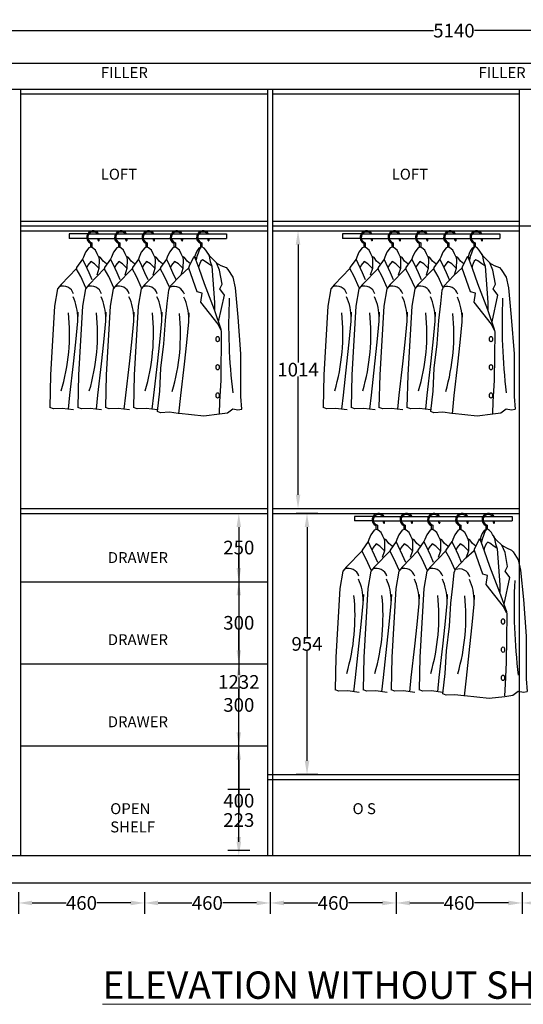
# Model space of a CAD drawing. Units: millimetres. Extents: x -472 to 16192, y -4730 to 4331.
# Tile 5 of 8: x 10934 to 12774, y -4730 to -1132. Entities that reach past the tile are written whole.
import ezdxf

# ---------------------------------------------------------------- set-up
doc = ezdxf.new("R2010")
doc.units = ezdxf.units.MM
doc.header["$MEASUREMENT"] = 0
for name, color, linetype, lineweight in [('A-ANNO-DIMS', 2, 'Continuous', 18), ('A-ANNO-TEXT', 6, 'Continuous', 18), ('A-ELEV', 7, 'Continuous', 25), ('A-FURN', 8, 'Continuous', 25)]:
    doc.layers.add(name, color=color, linetype=linetype, lineweight=lineweight)
doc.styles.get("Standard").update_dxf_attribs({"font": 'arial.ttf'})
doc.dimstyles.get("Standard").update_dxf_attribs({"dimtxt": 50, "dimasz": 50, "dimexe": 40, "dimexo": 40, "dimgap": 0.09, "dimtad": 0, "dimtih": 1, "dimtoh": 1, "dimdec": 0, "dimzin": 0, "dimdsep": 46, "dimtxsty": 'Standard', "dimcen": 0.09, "dimclrd": 1, "dimclre": 3, "dimclrt": 6, "dimadec": 0, "dimazin": 0, "dimtfac": 1, "dimtdec": 0, "dimtofl": 0, "dimtmove": 0, "dimatfit": 3, "dimfxl": 40, "dimfxlon": 1, "dimtolj": 1, "dimtzin": 0, "dimarcsym": 0})

# ---------------------------------------------------------------- blocks, each defined once
blk = doc.blocks.new('*D44')
at = {"layer": 'A-ANNO-DIMS', "color": 0, "lineweight": -2, "transparency": 16777216}
for p, q in [((9950.7, -1212.4), (9950.7, -1132.4)), ((15090.7, -1212.4), (15090.7, -1132.4)), ((10000.7, -1172.4), (12446, -1172.4)), ((15040.7, -1172.4), (12595.3, -1172.4))]:
    blk.add_line(p, q, dxfattribs=at)
at = {"layer": 'A-ANNO-DIMS', "color": 0, "transparency": 16777216}
for points in [[(10000.7, -1164.1), (10000.7, -1180.8), (9950.7, -1172.4)], [(15040.7, -1164.1), (15040.7, -1180.8), (15090.7, -1172.4)]]:
    blk.add_solid(points, dxfattribs=at)
at = {"layer": 'Defpoints', "color": 0, "transparency": 16777216}
for p in [(15090.7, -1172.4), (9950.7, -1290.9), (15090.7, -1290.9)]:
    blk.add_point(p, dxfattribs=at)
at = {"layer": 'A-ANNO-DIMS', "color": 0, "transparency": 16777216, "insert": (12520.7, -1172.4), "char_height": 50, "attachment_point": 5}
blk.add_mtext('\\A1;5140', dxfattribs=at)
blk = doc.blocks.new('*D54')
at = {"layer": 'A-ANNO-DIMS', "color": 0, "lineweight": -2, "transparency": 16777216}
for p, q in [((10929.7, -4319.4), (10929.7, -4399.4)), ((11389.7, -4319.4), (11389.7, -4399.4)), ((10979.7, -4359.4), (11103.4, -4359.4)), ((11339.7, -4359.4), (11215.9, -4359.4))]:
    blk.add_line(p, q, dxfattribs=at)
at = {"layer": 'A-ANNO-DIMS', "color": 0, "transparency": 16777216}
for points in [[(10979.7, -4351), (10979.7, -4367.7), (10929.7, -4359.4)], [(11339.7, -4351), (11339.7, -4367.7), (11389.7, -4359.4)]]:
    blk.add_solid(points, dxfattribs=at)
at = {"layer": 'Defpoints', "color": 0, "transparency": 16777216}
for p in [(10929.7, -4185.9), (11389.7, -4185.9), (11389.7, -4359.4)]:
    blk.add_point(p, dxfattribs=at)
at = {"layer": 'A-ANNO-DIMS', "color": 0, "transparency": 16777216, "insert": (11159.7, -4359.4), "char_height": 50, "attachment_point": 5}
blk.add_mtext('\\A1;460', dxfattribs=at)
blk = doc.blocks.new('*D55')
at = {"layer": 'A-ANNO-DIMS', "color": 0, "lineweight": -2, "transparency": 16777216}
for p, q in [((11389.7, -4319.4), (11389.7, -4399.4)), ((11849.7, -4319.4), (11849.7, -4399.4)), ((11439.7, -4359.4), (11563.4, -4359.4)), ((11799.7, -4359.4), (11675.9, -4359.4))]:
    blk.add_line(p, q, dxfattribs=at)
at = {"layer": 'A-ANNO-DIMS', "color": 0, "transparency": 16777216}
for points in [[(11439.7, -4351), (11439.7, -4367.7), (11389.7, -4359.4)], [(11799.7, -4351), (11799.7, -4367.7), (11849.7, -4359.4)]]:
    blk.add_solid(points, dxfattribs=at)
at = {"layer": 'Defpoints', "color": 0, "transparency": 16777216}
for p in [(11389.7, -4185.9), (11849.7, -4185.9), (11849.7, -4359.4)]:
    blk.add_point(p, dxfattribs=at)
at = {"layer": 'A-ANNO-DIMS', "color": 0, "transparency": 16777216, "insert": (11619.7, -4359.4), "char_height": 50, "attachment_point": 5}
blk.add_mtext('\\A1;460', dxfattribs=at)
blk = doc.blocks.new('*D56')
at = {"layer": 'A-ANNO-DIMS', "color": 0, "lineweight": -2, "transparency": 16777216}
for p, q in [((11849.7, -4319.4), (11849.7, -4399.4)), ((12309.7, -4319.4), (12309.7, -4399.4)), ((11899.7, -4359.4), (12023.4, -4359.4)), ((12259.7, -4359.4), (12135.9, -4359.4))]:
    blk.add_line(p, q, dxfattribs=at)
at = {"layer": 'A-ANNO-DIMS', "color": 0, "transparency": 16777216}
for points in [[(11899.7, -4351), (11899.7, -4367.7), (11849.7, -4359.4)], [(12259.7, -4351), (12259.7, -4367.7), (12309.7, -4359.4)]]:
    blk.add_solid(points, dxfattribs=at)
at = {"layer": 'Defpoints', "color": 0, "transparency": 16777216}
for p in [(11849.7, -4185.9), (12309.7, -4185.9), (12309.7, -4359.4)]:
    blk.add_point(p, dxfattribs=at)
at = {"layer": 'A-ANNO-DIMS', "color": 0, "transparency": 16777216, "insert": (12079.7, -4359.4), "char_height": 50, "attachment_point": 5}
blk.add_mtext('\\A1;460', dxfattribs=at)
blk = doc.blocks.new('*D57')
at = {"layer": 'A-ANNO-DIMS', "color": 0, "lineweight": -2, "transparency": 16777216}
for p, q in [((12309.7, -4319.4), (12309.7, -4399.4)), ((12769.7, -4319.4), (12769.7, -4399.4)), ((12359.7, -4359.4), (12483.4, -4359.4)), ((12719.7, -4359.4), (12595.9, -4359.4))]:
    blk.add_line(p, q, dxfattribs=at)
at = {"layer": 'A-ANNO-DIMS', "color": 0, "transparency": 16777216}
for points in [[(12359.7, -4351), (12359.7, -4367.7), (12309.7, -4359.4)], [(12719.7, -4351), (12719.7, -4367.7), (12769.7, -4359.4)]]:
    blk.add_solid(points, dxfattribs=at)
at = {"layer": 'Defpoints', "color": 0, "transparency": 16777216}
for p in [(12309.7, -4185.9), (12769.7, -4185.9), (12769.7, -4359.4)]:
    blk.add_point(p, dxfattribs=at)
at = {"layer": 'A-ANNO-DIMS', "color": 0, "transparency": 16777216, "insert": (12539.7, -4359.4), "char_height": 50, "attachment_point": 5}
blk.add_mtext('\\A1;460', dxfattribs=at)
blk = doc.blocks.new('*D58')
at = {"layer": 'A-ANNO-DIMS', "color": 0, "lineweight": -2, "transparency": 16777216}
for p, q in [((12769.7, -4319.4), (12769.7, -4399.4)), ((13229.7, -4319.4), (13229.7, -4399.4)), ((12819.7, -4359.4), (12943.4, -4359.4)), ((13179.7, -4359.4), (13055.9, -4359.4))]:
    blk.add_line(p, q, dxfattribs=at)
at = {"layer": 'A-ANNO-DIMS', "color": 0, "transparency": 16777216}
for points in [[(12819.7, -4351), (12819.7, -4367.7), (12769.7, -4359.4)], [(13179.7, -4351), (13179.7, -4367.7), (13229.7, -4359.4)]]:
    blk.add_solid(points, dxfattribs=at)
at = {"layer": 'Defpoints', "color": 0, "transparency": 16777216}
for p in [(12769.7, -4185.9), (13229.7, -4185.9), (13229.7, -4359.4)]:
    blk.add_point(p, dxfattribs=at)
at = {"layer": 'A-ANNO-DIMS', "color": 0, "transparency": 16777216, "insert": (12999.7, -4359.4), "char_height": 50, "attachment_point": 5}
blk.add_mtext('\\A1;460', dxfattribs=at)
blk = doc.blocks.new('*D73')
at = {"layer": 'A-ANNO-DIMS', "color": 0, "lineweight": -2, "transparency": 16777216}
for p, q in [((11911.1, -1903.9), (11991.1, -1903.9)), ((11951.1, -1953.9), (11951.1, -2385.3)), ((11951.1, -2867.9), (11951.1, -2436.5)), ((11911.1, -2917.9), (11991.1, -2917.9))]:
    blk.add_line(p, q, dxfattribs=at)
at = {"layer": 'A-ANNO-DIMS', "color": 0, "transparency": 16777216}
for points in [[(11942.8, -1953.9), (11959.5, -1953.9), (11951.1, -1903.9)], [(11942.8, -2867.9), (11959.5, -2867.9), (11951.1, -2917.9)]]:
    blk.add_solid(points, dxfattribs=at)
at = {"layer": 'Defpoints', "color": 0, "transparency": 16777216}
for p in [(11851.5, -1903.9), (11851.5, -2917.9), (11951.1, -2917.9)]:
    blk.add_point(p, dxfattribs=at)
at = {"layer": 'A-ANNO-DIMS', "color": 0, "transparency": 16777216, "insert": (11951.1, -2410.9), "char_height": 50, "attachment_point": 5}
blk.add_mtext('\\A1;1014', dxfattribs=at)
blk = doc.blocks.new('*D74')
at = {"layer": 'A-ANNO-DIMS', "color": 0, "lineweight": -2, "transparency": 16777216}
for p, q in [((12023.9, -2935.9), (11943.9, -2935.9)), ((11983.9, -2985.9), (11983.9, -3387.3)), ((11983.9, -3839.9), (11983.9, -3438.5)), ((12023.9, -3889.9), (11943.9, -3889.9))]:
    blk.add_line(p, q, dxfattribs=at)
at = {"layer": 'A-ANNO-DIMS', "color": 0, "transparency": 16777216}
for points in [[(11975.6, -2985.9), (11992.3, -2985.9), (11983.9, -2935.9)], [(11975.6, -3839.9), (11992.3, -3839.9), (11983.9, -3889.9)]]:
    blk.add_solid(points, dxfattribs=at)
at = {"layer": 'Defpoints', "color": 0, "transparency": 16777216}
for p in [(12121.2, -2935.9), (11983.9, -3889.9), (12103.5, -3889.9)]:
    blk.add_point(p, dxfattribs=at)
at = {"layer": 'A-ANNO-DIMS', "color": 0, "transparency": 16777216, "insert": (11983.9, -3412.9), "char_height": 50, "attachment_point": 5}
blk.add_mtext('\\A1;954', dxfattribs=at)
blk = doc.blocks.new('*D82')
at = {"layer": 'A-ANNO-DIMS', "color": 0, "lineweight": -2, "transparency": 16777216}
for p, q in [((11733.2, -3785.9), (11774.7, -3785.9)), ((11734.7, -3835.9), (11734.7, -3960.3)), ((11734.7, -4135.9), (11734.7, -4011.5)), ((11733.2, -4185.9), (11774.7, -4185.9))]:
    blk.add_line(p, q, dxfattribs=at)
at = {"layer": 'A-ANNO-DIMS', "color": 0, "transparency": 16777216}
for points in [[(11726.4, -3835.9), (11743, -3835.9), (11734.7, -3785.9)], [(11726.4, -4135.9), (11743, -4135.9), (11734.7, -4185.9)]]:
    blk.add_solid(points, dxfattribs=at)
at = {"layer": 'Defpoints', "color": 0, "transparency": 16777216}
for p in [(11693.2, -3785.9), (11734.7, -3785.9), (11693.2, -4185.9)]:
    blk.add_point(p, dxfattribs=at)
at = {"layer": 'A-ANNO-DIMS', "color": 0, "transparency": 16777216, "insert": (11734.7, -3985.9), "char_height": 50, "attachment_point": 5}
blk.add_mtext('\\A1;400', dxfattribs=at)
blk = doc.blocks.new('*D83')
at = {"layer": 'A-ANNO-DIMS', "color": 0, "lineweight": -2, "transparency": 16777216}
for p, q in [((11734.7, -3485.9), (11774.7, -3485.9)), ((11734.7, -3535.9), (11734.7, -3610.3)), ((11734.7, -3735.9), (11734.7, -3661.5)), ((11733.2, -3785.9), (11774.7, -3785.9))]:
    blk.add_line(p, q, dxfattribs=at)
at = {"layer": 'A-ANNO-DIMS', "color": 0, "transparency": 16777216}
for points in [[(11726.4, -3535.9), (11743, -3535.9), (11734.7, -3485.9)], [(11726.4, -3735.9), (11743, -3735.9), (11734.7, -3785.9)]]:
    blk.add_solid(points, dxfattribs=at)
at = {"layer": 'Defpoints', "color": 0, "transparency": 16777216}
for p in [(11734.7, -3485.9), (11734.7, -3485.9), (11693.2, -3785.9)]:
    blk.add_point(p, dxfattribs=at)
at = {"layer": 'A-ANNO-DIMS', "color": 0, "transparency": 16777216, "insert": (11734.7, -3635.9), "char_height": 50, "attachment_point": 5}
blk.add_mtext('\\A1;300', dxfattribs=at)
blk = doc.blocks.new('*D84')
at = {"layer": 'A-ANNO-DIMS', "color": 0, "lineweight": -2, "transparency": 16777216}
for p, q in [((11734.7, -3185.9), (11774.7, -3185.9)), ((11734.7, -3235.9), (11734.7, -3310.3)), ((11734.7, -3435.9), (11734.7, -3361.5)), ((11734.7, -3485.9), (11774.7, -3485.9))]:
    blk.add_line(p, q, dxfattribs=at)
at = {"layer": 'A-ANNO-DIMS', "color": 0, "transparency": 16777216}
for points in [[(11726.4, -3235.9), (11743, -3235.9), (11734.7, -3185.9)], [(11726.4, -3435.9), (11743, -3435.9), (11734.7, -3485.9)]]:
    blk.add_solid(points, dxfattribs=at)
at = {"layer": 'Defpoints', "color": 0, "transparency": 16777216}
for p in [(11734.7, -3185.9), (11734.7, -3185.9), (11734.7, -3485.9)]:
    blk.add_point(p, dxfattribs=at)
at = {"layer": 'A-ANNO-DIMS', "color": 0, "transparency": 16777216, "insert": (11734.7, -3335.9), "char_height": 50, "attachment_point": 5}
blk.add_mtext('\\A1;300', dxfattribs=at)
blk = doc.blocks.new('*D85')
at = {"layer": 'A-ANNO-DIMS', "color": 0, "lineweight": -2, "transparency": 16777216}
for p, q in [((11734.7, -2935.9), (11774.7, -2935.9)), ((11734.7, -2985.9), (11734.7, -3035.3)), ((11734.7, -3135.9), (11734.7, -3086.5)), ((11734.7, -3185.9), (11774.7, -3185.9))]:
    blk.add_line(p, q, dxfattribs=at)
at = {"layer": 'A-ANNO-DIMS', "color": 0, "transparency": 16777216}
for points in [[(11726.4, -2985.9), (11743, -2985.9), (11734.7, -2935.9)], [(11726.4, -3135.9), (11743, -3135.9), (11734.7, -3185.9)]]:
    blk.add_solid(points, dxfattribs=at)
at = {"layer": 'Defpoints', "color": 0, "transparency": 16777216}
for p in [(11734.7, -2935.9), (11734.7, -2935.9), (11734.7, -3185.9)]:
    blk.add_point(p, dxfattribs=at)
at = {"layer": 'A-ANNO-DIMS', "color": 0, "transparency": 16777216, "insert": (11734.7, -3060.9), "char_height": 50, "attachment_point": 5}
blk.add_mtext('\\A1;250', dxfattribs=at)
blk = doc.blocks.new('*D86')
at = {"layer": 'A-ANNO-DIMS', "color": 0, "lineweight": -2, "transparency": 16777216}
for p, q in [((11734.7, -2935.9), (11774.7, -2935.9)), ((11734.7, -2985.9), (11734.7, -3526.3)), ((11734.7, -4117.9), (11734.7, -3577.5)), ((11774.7, -4167.9), (11694.7, -4167.9))]:
    blk.add_line(p, q, dxfattribs=at)
at = {"layer": 'A-ANNO-DIMS', "color": 0, "transparency": 16777216}
for points in [[(11726.4, -2985.9), (11743, -2985.9), (11734.7, -2935.9)], [(11726.4, -4117.9), (11743, -4117.9), (11734.7, -4167.9)]]:
    blk.add_solid(points, dxfattribs=at)
at = {"layer": 'Defpoints', "color": 0, "transparency": 16777216}
for p in [(11734.7, -2935.9), (11734.7, -4167.9), (14004.4, -4167.9)]:
    blk.add_point(p, dxfattribs=at)
at = {"layer": 'A-ANNO-DIMS', "color": 0, "transparency": 16777216, "insert": (11734.7, -3551.9), "char_height": 50, "attachment_point": 5}
blk.add_mtext('\\A1;1232', dxfattribs=at)
blk = doc.blocks.new('*D87')
at = {"layer": 'A-ANNO-DIMS', "color": 0, "lineweight": -2, "transparency": 16777216}
for p, q in [((11774.7, -3944.9), (11694.7, -3944.9)), ((11734.7, -3994.9), (11734.7, -4030.8)), ((11734.7, -4117.9), (11734.7, -4082)), ((11774.7, -4167.9), (11694.7, -4167.9))]:
    blk.add_line(p, q, dxfattribs=at)
at = {"layer": 'A-ANNO-DIMS', "color": 0, "transparency": 16777216}
for points in [[(11726.4, -3994.9), (11743, -3994.9), (11734.7, -3944.9)], [(11726.4, -4117.9), (11743, -4117.9), (11734.7, -4167.9)]]:
    blk.add_solid(points, dxfattribs=at)
at = {"layer": 'Defpoints', "color": 0, "transparency": 16777216}
for p in [(11734.7, -3944.9), (13999.1, -3944.9), (14004.4, -4167.9)]:
    blk.add_point(p, dxfattribs=at)
at = {"layer": 'A-ANNO-DIMS', "color": 0, "transparency": 16777216, "insert": (11734.7, -4056.4), "char_height": 50, "attachment_point": 5}
blk.add_mtext('\\A1;223', dxfattribs=at)
blk = doc.blocks.new('7')
for p, q in [((3901.77, 12903.37), (3898.37, 12903.37)), ((3898.37, 12903.37), (3898.37, 12902.56)), ((3901.6, 12902.56), (3898.37, 12902.56)), ((3901.81, 12902.56), (3906.72, 12902.56)), ((3902.01, 12903.37), (3906.88, 12903.37)), ((3902.55, 12901.75), (3902.55, 12900.89)), ((3903.8, 12903.37), (3905.4, 12903.37)), ((3906.93, 12902.56), (3911.77, 12902.56)), ((3907.13, 12903.37), (3911.93, 12903.37)), ((3907.67, 12901.75), (3907.67, 12900.89)), ((3911.97, 12902.56), (3916.93, 12902.56)), ((3912.18, 12903.37), (3917.09, 12903.37)), ((3912.72, 12901.75), (3912.72, 12900.89)), ((3917.13, 12902.56), (3921.77, 12902.56)), ((3917.33, 12903.37), (3921.94, 12903.37)), ((3917.87, 12901.75), (3917.87, 12900.92)), ((3921.98, 12902.56), (3927.26, 12902.56)), ((3922.18, 12903.37), (3927.26, 12903.37)), ((3922.72, 12901.75), (3922.72, 12901.02)), ((3927.26, 12903.37), (3927.26, 12902.56)), ((3901.37, 12900), (3900.98, 12899.12)), ((3901.99, 12900.85), (3901.37, 12900)), ((3902.38, 12900.93), (3901.99, 12900.85)), ((3902.35, 12900.89), (3902.35, 12901.61)), ((3902.69, 12900.85), (3902.38, 12900.93)), ((3903.23, 12900.39), (3902.69, 12900.85)), ((3903.54, 12899.74), (3903.23, 12900.39)), ((3906.51, 12900), (3906.12, 12899.12)), ((3907.13, 12900.85), (3906.51, 12900)), ((3907.52, 12900.93), (3907.13, 12900.85)), ((3907.47, 12900.89), (3907.47, 12901.61)), ((3907.83, 12900.85), (3907.52, 12900.93)), ((3908.37, 12900.39), (3907.83, 12900.85)), ((3908.68, 12899.74), (3908.37, 12900.39)), ((3911.62, 12900), (3911.24, 12899.12)), ((3912.25, 12900.85), (3911.62, 12900)), ((3912.63, 12900.93), (3912.25, 12900.85)), ((3912.51, 12900.89), (3912.51, 12901.61)), ((3912.94, 12900.85), (3912.63, 12900.93)), ((3913.49, 12900.39), (3912.94, 12900.85)), ((3913.8, 12899.74), (3913.49, 12900.39)), ((3916.76, 12900), (3916.38, 12899.12)), ((3917.39, 12900.85), (3916.76, 12900)), ((3917.77, 12900.93), (3917.39, 12900.85)), ((3917.67, 12900.91), (3917.67, 12901.61)), ((3918.08, 12900.85), (3917.77, 12900.93)), ((3918.63, 12900.39), (3918.08, 12900.85)), ((3918.94, 12899.74), (3918.63, 12900.39)), ((3921.8, 12900.21), (3921.6, 12899.78)), ((3922.16, 12900.76), (3921.8, 12900.21)), ((3922.35, 12900.7), (3922.02, 12899.87)), ((3922.57, 12901.03), (3922.16, 12900.76)), ((3922.57, 12901.03), (3922.35, 12900.7)), ((3922.52, 12901), (3922.52, 12901.61)), ((3922.75, 12901), (3922.57, 12901.03)), ((3923.13, 12900.79), (3922.75, 12901)), ((3923.47, 12900.38), (3923.13, 12900.79)), ((3923.71, 12900.01), (3923.47, 12900.38)), ((3924, 12899.6), (3923.71, 12900.01)), ((3900.85, 12898.74), (3899.74, 12897.19)), ((3900.98, 12899.12), (3900.85, 12898.73)), ((3901.25, 12897.93), (3900.85, 12898.74)), ((3902.33, 12898.32), (3901.78, 12897.67)), ((3903.03, 12897.88), (3902.33, 12898.32)), ((3903.78, 12899.26), (3903.54, 12899.74)), ((3904.15, 12899.04), (3903.78, 12899.26)), ((3903.78, 12899.26), (3903.89, 12898.71)), ((3903.89, 12898.71), (3903.85, 12897.04)), ((3904.63, 12898.37), (3904.15, 12899.04)), ((3905.24, 12897.91), (3904.63, 12898.37)), ((3905.99, 12898.74), (3904.88, 12897.19)), ((3906.12, 12899.12), (3905.99, 12898.73)), ((3906.39, 12897.93), (3905.99, 12898.74)), ((3907.47, 12898.32), (3906.92, 12897.67)), ((3908.17, 12897.88), (3907.47, 12898.32)), ((3908.92, 12899.26), (3908.68, 12899.74)), ((3909.29, 12899.04), (3908.92, 12899.26)), ((3908.92, 12899.26), (3909.03, 12898.71)), ((3909.03, 12898.71), (3908.99, 12897.04)), ((3909.77, 12898.37), (3909.29, 12899.04)), ((3910.38, 12897.91), (3909.77, 12898.37)), ((3911.1, 12898.74), (3909.99, 12897.19)), ((3911.51, 12897.93), (3911.1, 12898.74)), ((3911.24, 12899.12), (3911.11, 12898.73)), ((3912.58, 12898.32), (3912.04, 12897.67)), ((3913.28, 12897.88), (3912.58, 12898.32)), ((3914.03, 12899.26), (3913.8, 12899.74)), ((3914.4, 12899.04), (3914.03, 12899.26)), ((3914.03, 12899.26), (3914.14, 12898.71)), ((3914.14, 12898.71), (3914.11, 12897.04)), ((3914.88, 12898.37), (3914.4, 12899.04)), ((3915.5, 12897.91), (3914.88, 12898.37)), ((3916.24, 12898.74), (3915.13, 12897.19)), ((3916.65, 12897.93), (3916.24, 12898.74)), ((3916.38, 12899.12), (3916.25, 12898.73)), ((3917.72, 12898.32), (3917.18, 12897.67)), ((3918.42, 12897.88), (3917.72, 12898.32)), ((3919.17, 12899.26), (3918.94, 12899.74)), ((3919.54, 12899.04), (3919.17, 12899.26)), ((3919.17, 12899.26), (3919.28, 12898.71)), ((3919.28, 12898.71), (3919.25, 12897.04)), ((3920.02, 12898.37), (3919.54, 12899.04)), ((3920.64, 12897.91), (3920.02, 12898.37)), ((3920.43, 12897.51), (3920.79, 12898.19)), ((3920.79, 12898.19), (3921.19, 12898.97)), ((3921.19, 12898.97), (3921.35, 12899.23)), ((3921.3, 12899.16), (3921.61, 12898.57)), ((3921.35, 12899.23), (3921.7, 12898.97)), ((3921.6, 12899.78), (3921.4, 12899.16)), ((3921.61, 12898.57), (3922.15, 12897.07)), ((3921.66, 12898.64), (3921.65, 12898.56)), ((3921.8, 12899.21), (3921.66, 12898.64)), ((3921.7, 12898.97), (3921.75, 12898.95)), ((3922.02, 12899.87), (3921.8, 12899.21)), ((3922.55, 12898.4), (3922.33, 12897.95)), ((3922.82, 12898.65), (3922.55, 12898.4)), ((3923.17, 12898.44), (3922.82, 12898.65)), ((3923.96, 12897.86), (3923.17, 12898.44)), ((3924.38, 12899.09), (3923.92, 12899.61)), ((3924, 12899.6), (3924.26, 12898.31)), ((3924.26, 12898.31), (3924.56, 12897.43)), ((3925.4, 12898.1), (3924.38, 12899.09)), ((3899.74, 12897.04), (3896.88, 12894.08)), ((3900.49, 12895.54), (3899.68, 12897.02)), ((3899.74, 12897.19), (3899.74, 12897.04)), ((3902.03, 12896.26), (3901.25, 12897.93)), ((3901.78, 12897.67), (3901.59, 12897.2)), ((3904.88, 12897.04), (3902.02, 12894.08)), ((3903.88, 12897.03), (3903.03, 12897.88)), ((3903.85, 12897.04), (3903.46, 12895.81)), ((3905.63, 12895.54), (3904.82, 12897.02)), ((3904.88, 12897.19), (3904.88, 12897.04)), ((3907.17, 12896.26), (3906.39, 12897.93)), ((3906.92, 12897.67), (3906.73, 12897.2)), ((3909.99, 12897.04), (3907.14, 12894.08)), ((3909.02, 12897.03), (3908.17, 12897.88)), ((3908.99, 12897.04), (3908.6, 12895.81)), ((3910.75, 12895.54), (3909.93, 12897.02)), ((3909.99, 12897.19), (3909.99, 12897.04)), ((3912.29, 12896.26), (3911.51, 12897.93)), ((3912.04, 12897.67), (3911.85, 12897.2)), ((3915.13, 12897.04), (3912.28, 12894.08)), ((3914.13, 12897.03), (3913.28, 12897.88)), ((3914.11, 12897.04), (3913.72, 12895.81)), ((3915.89, 12895.54), (3915.07, 12897.02)), ((3915.13, 12897.19), (3915.13, 12897.04)), ((3917.43, 12896.26), (3916.65, 12897.93)), ((3917.18, 12897.67), (3916.99, 12897.2)), ((3919.27, 12897.03), (3918.42, 12897.88)), ((3918.8, 12895.75), (3920.32, 12897.13)), ((3919.25, 12897.04), (3918.86, 12895.81)), ((3920.32, 12897.13), (3920.43, 12897.51)), ((3921.88, 12892.78), (3920.35, 12897.12)), ((3922.18, 12897.46), (3922.13, 12897.29)), ((3922.15, 12897.07), (3923.16, 12894.25)), ((3922.33, 12897.95), (3922.18, 12897.46)), ((3924.48, 12897.51), (3923.96, 12897.86)), ((3924.56, 12897.43), (3925.04, 12890.79)), ((3925.37, 12898.1), (3926.22, 12897.58)), ((3925.98, 12896.74), (3925.4, 12898.1)), ((3926.43, 12894.14), (3925.98, 12896.74)), ((3926.22, 12897.58), (3927.16, 12897.19)), ((3927.16, 12897.19), (3927.49, 12896.83)), ((3927.49, 12896.83), (3928.42, 12895.42)), ((3901.42, 12893.5), (3900.49, 12895.54)), ((3902.61, 12894.93), (3902.03, 12896.26)), ((3906.56, 12893.5), (3905.63, 12895.54)), ((3907.75, 12894.93), (3907.17, 12896.26)), ((3911.68, 12893.5), (3910.75, 12895.54)), ((3912.86, 12894.93), (3912.29, 12896.26)), ((3916.82, 12893.5), (3915.89, 12895.54)), ((3916.93, 12893.82), (3918.8, 12895.75)), ((3918, 12894.93), (3917.43, 12896.26)), ((3928.42, 12895.42), (3928.82, 12893.49)), ((3896.21, 12893.3), (3895.68, 12890.13)), ((3896.88, 12894.08), (3896.21, 12893.3)), ((3901.35, 12893.3), (3900.82, 12890.13)), ((3902.02, 12894.08), (3901.35, 12893.3)), ((3906.47, 12893.3), (3905.93, 12890.13)), ((3907.14, 12894.08), (3906.47, 12893.3)), ((3911.61, 12893.3), (3911.07, 12890.13)), ((3912.28, 12894.08), (3911.61, 12893.3)), ((3916.38, 12890.58), (3916.66, 12893.06)), ((3916.66, 12893.06), (3916.93, 12893.82)), ((3922.78, 12892.51), (3921.88, 12892.78)), ((3923.16, 12894.25), (3924.99, 12889.48)), ((3926.01, 12893.3), (3926.43, 12894.14)), ((3926.86, 12892.12), (3926.01, 12893.3)), ((3928.82, 12893.49), (3929.34, 12888.11)), ((3922.52, 12890.85), (3922.78, 12892.51)), ((3925.8, 12887.26), (3926.86, 12892.12)), ((3895.68, 12890.13), (3894.93, 12877.55)), ((3900.82, 12890.13), (3900.07, 12877.55)), ((3905.93, 12890.13), (3905.19, 12877.55)), ((3911.07, 12890.13), (3910.33, 12877.55)), ((3916.04, 12887.47), (3916.38, 12890.58)), ((3925.72, 12886.84), (3922.52, 12890.85)), ((3924.99, 12889.48), (3926.22, 12885.93)), ((3925.04, 12890.79), (3925.04, 12889.46)), ((3899.6, 12883.53), (3899.96, 12887.35)), ((3899.96, 12887.35), (3900.04, 12889.01)), ((3904.74, 12883.53), (3905.1, 12887.35)), ((3905.1, 12887.35), (3905.18, 12889.01)), ((3909.86, 12883.53), (3910.22, 12887.35)), ((3910.22, 12887.35), (3910.29, 12889.01)), ((3915, 12883.53), (3915.36, 12887.35)), ((3915.36, 12887.35), (3915.43, 12889.01)), ((3915.76, 12883.2), (3916.04, 12887.47)), ((3920.32, 12887.26), (3920.4, 12888.92)), ((3929.34, 12888.11), (3929.84, 12881.39)), ((3919.96, 12883.44), (3920.32, 12887.26)), ((3926.26, 12885.67), (3925.72, 12886.84)), ((3926.22, 12885.93), (3926.3, 12885.33)), ((3926.3, 12885.33), (3926.19, 12876.54)), ((3899.17, 12879.56), (3899.6, 12883.53)), ((3904.31, 12879.56), (3904.74, 12883.53)), ((3909.43, 12879.56), (3909.86, 12883.53)), ((3914.57, 12879.56), (3915, 12883.53)), ((3915.21, 12878.72), (3915.76, 12883.2)), ((3919.53, 12879.47), (3919.96, 12883.44)), ((3929.84, 12881.39), (3929.84, 12873.56)), ((3898.52, 12873.79), (3899.17, 12879.56)), ((3903.66, 12873.79), (3904.31, 12879.56)), ((3908.78, 12873.79), (3909.43, 12879.56)), ((3913.92, 12873.79), (3914.57, 12879.56)), ((3915, 12874.51), (3915.21, 12878.72)), ((3918.88, 12873.7), (3919.53, 12879.47)), ((3894.93, 12877.55), (3894.8, 12871.54)), ((3900.07, 12877.55), (3899.94, 12871.54)), ((3905.19, 12877.55), (3905.06, 12871.54)), ((3910.33, 12877.55), (3910.2, 12871.54)), ((3926.19, 12876.54), (3925.98, 12872.58)), ((3898.24, 12871.2), (3898.52, 12873.79)), ((3903.38, 12871.2), (3903.66, 12873.79)), ((3908.49, 12871.2), (3908.78, 12873.79)), ((3913.63, 12871.2), (3913.92, 12873.79)), ((3914.56, 12870.79), (3915, 12874.51)), ((3918.52, 12870.38), (3918.88, 12873.7)), ((3929.84, 12873.56), (3930.02, 12871.22)), ((3895.48, 12871.28), (3894.8, 12871.54)), ((3897.11, 12871.35), (3895.48, 12871.28)), ((3899.2, 12871.07), (3897.11, 12871.35)), ((3900.62, 12871.28), (3899.94, 12871.54)), ((3902.25, 12871.35), (3900.62, 12871.28)), ((3904.34, 12871.07), (3902.25, 12871.35)), ((3905.74, 12871.28), (3905.06, 12871.54)), ((3907.37, 12871.35), (3905.74, 12871.28)), ((3909.45, 12871.07), (3907.37, 12871.35)), ((3910.88, 12871.28), (3910.2, 12871.54)), ((3912.51, 12871.35), (3910.88, 12871.28)), ((3914.59, 12871.07), (3912.51, 12871.35)), ((3925.98, 12872.58), (3925.91, 12870.44)), ((3927.43, 12870.57), (3928.42, 12871.3)), ((3928.42, 12871.3), (3929.35, 12871.09)), ((3929.35, 12871.09), (3930.07, 12871.23)), ((3915.15, 12870.57), (3914.56, 12870.79)), ((3916.78, 12870.64), (3915.15, 12870.57)), ((3918.41, 12870.42), (3916.78, 12870.64)), ((3918.56, 12870.49), (3923.07, 12869.98)), ((3923.07, 12869.98), (3925.95, 12870.34)), ((3925.95, 12870.34), (3927.43, 12870.57))]:
    blk.add_line(p, q)
for centre, radius, start, end in [((3902.79, 12902.74), 1.19, 31.4138, 165.4823), ((3902.79, 12902.74), 0.991, 38.898, 165.4823), ((3907.9, 12902.74), 1.19, 31.4138, 165.4823), ((3907.9, 12902.74), 0.991, 38.898, 165.4823), ((3912.95, 12902.74), 1.19, 31.4138, 165.4823), ((3912.95, 12902.74), 0.991, 38.898, 165.4823), ((3918.11, 12902.74), 1.19, 31.4138, 165.4823), ((3918.11, 12902.74), 0.991, 38.898, 165.4823), ((3922.95, 12902.74), 1.19, 31.4138, 165.4823), ((3922.95, 12902.74), 0.991, 38.898, 165.4823), ((3902.81, 12902.74), 1.22, 165.4823, 247.8669), ((3902.81, 12902.74), 1.02, 165.4823, 255.3823), ((3902.7, 12902.33), 0.991, 354.9774, 12.9498), ((3903.79, 12902.23), 0.102, 171.8983, 358.0565), ((3902.7, 12902.33), 1.19, 354.9774, 10.7201), ((3907.93, 12902.74), 1.22, 165.4823, 247.8669), ((3907.93, 12902.74), 1.02, 165.4823, 255.3823), ((3907.81, 12902.33), 0.991, 354.9774, 12.9498), ((3908.9, 12902.23), 0.102, 171.8983, 358.0565), ((3907.81, 12902.33), 1.19, 354.9774, 10.7201), ((3912.97, 12902.74), 1.22, 165.4823, 247.8669), ((3912.97, 12902.74), 1.02, 165.4823, 255.3823), ((3912.86, 12902.33), 0.991, 354.9774, 12.9498), ((3913.95, 12902.23), 0.102, 171.8983, 358.0565), ((3912.86, 12902.33), 1.19, 354.9774, 10.7201), ((3918.13, 12902.74), 1.22, 165.4823, 247.8669), ((3918.13, 12902.74), 1.02, 165.4823, 255.3823), ((3918.02, 12902.33), 0.991, 354.9774, 12.9498), ((3919.11, 12902.23), 0.102, 171.8983, 358.0565), ((3918.02, 12902.33), 1.19, 354.9774, 10.7201), ((3922.98, 12902.74), 1.22, 165.4823, 247.8669), ((3922.98, 12902.74), 1.02, 165.4823, 255.3823), ((3922.87, 12902.33), 0.991, 354.9774, 12.9498), ((3923.95, 12902.23), 0.102, 171.8983, 358.0565), ((3922.87, 12902.33), 1.19, 354.9774, 10.7201), ((3897.26, 12891.85), 1.97, 15.7523, 111.1565), ((3902.4, 12891.85), 1.97, 15.7523, 111.1565), ((3907.51, 12891.85), 1.97, 15.7523, 111.1565), ((3912.65, 12891.85), 1.97, 15.7523, 111.1565), ((3917.62, 12891.76), 1.97, 15.7523, 111.1565), ((3890.5, 12887.86), 9.47, 359.9116, 24.988), ((3895.64, 12887.86), 9.47, 359.9116, 24.988), ((3900.76, 12887.86), 9.47, 359.9116, 24.988), ((3905.9, 12887.86), 9.47, 359.9116, 24.988), ((3910.86, 12887.76), 9.47, 359.9116, 24.988), ((4029.55, 12886.77), 101.91, 177.2767, 187.0811), ((3861.53, 12885.02), 36.92, 343.5409, 5.9886), ((3866.67, 12885.02), 36.92, 343.5409, 5.9886), ((3876.93, 12885.02), 36.92, 343.5409, 5.9886), ((3881.89, 12884.93), 36.92, 343.5409, 5.9886)]:
    blk.add_arc(centre, radius, start, end)
for centre in [(3925.62, 12884.08), (3925.62, 12878.91), (3925.62, 12873.74)]:
    blk.add_ellipse(centre, major_axis=(0, 0.503), ratio=0.580645)
blk = doc.blocks.new('*D100')
at = {"layer": 'A-ANNO-DIMS', "color": 1, "lineweight": -2, "transparency": 16777216}
for p, q in [((16116.7, -1835.9), (16116.7, -1785.9)), ((16116.7, -2035.9), (16116.7, -2085.9))]:
    blk.add_line(p, q, dxfattribs=at)
at = {"layer": 'A-ANNO-DIMS', "color": 3, "lineweight": -2, "transparency": 16777216}
for p, q in [((16076.7, -1885.9), (16156.7, -1885.9)), ((16076.7, -1985.9), (16156.7, -1985.9))]:
    blk.add_line(p, q, dxfattribs=at)
at = {"layer": 'A-ANNO-DIMS', "color": 1, "transparency": 16777216}
for points in [[(16108.3, -1835.9), (16125, -1835.9), (16116.7, -1885.9)], [(16108.3, -2035.9), (16125, -2035.9), (16116.7, -1985.9)]]:
    blk.add_solid(points, dxfattribs=at)
at = {"layer": 'Defpoints', "color": 0, "transparency": 16777216}
for p in [(5309, -1885.9), (5209, -1985.9), (16116.7, -1985.9)]:
    blk.add_point(p, dxfattribs=at)
at = {"layer": 'A-ANNO-DIMS', "color": 6, "transparency": 16777216, "insert": (16116.7, -1935.9), "char_height": 50, "attachment_point": 5}
blk.add_mtext('\\A1;100', dxfattribs=at)
blk = doc.blocks.new('*D101')
at = {"layer": 'A-ANNO-DIMS', "color": 3, "lineweight": -2, "transparency": 16777216}
for p, q in [((16076.7, -1985.9), (16156.7, -1985.9)), ((16076.7, -3535.9), (16156.7, -3535.9))]:
    blk.add_line(p, q, dxfattribs=at)
at = {"layer": 'A-ANNO-DIMS', "color": 1, "lineweight": -2, "transparency": 16777216}
for p, q in [((16116.7, -2035.9), (16116.7, -2735.3)), ((16116.7, -3485.9), (16116.7, -2786.5))]:
    blk.add_line(p, q, dxfattribs=at)
at = {"layer": 'A-ANNO-DIMS', "color": 1, "transparency": 16777216}
for points in [[(16108.3, -2035.9), (16125, -2035.9), (16116.7, -1985.9)], [(16108.3, -3485.9), (16125, -3485.9), (16116.7, -3535.9)]]:
    blk.add_solid(points, dxfattribs=at)
at = {"layer": 'Defpoints', "color": 0, "transparency": 16777216}
for p in [(5209, -1985.9), (5209, -3535.9), (16116.7, -3535.9)]:
    blk.add_point(p, dxfattribs=at)
at = {"layer": 'A-ANNO-DIMS', "color": 6, "transparency": 16777216, "insert": (16116.7, -2760.9), "char_height": 50, "attachment_point": 5}
blk.add_mtext('\\A1;1550', dxfattribs=at)
blk = doc.blocks.new('*D102')
at = {"layer": 'A-ANNO-DIMS', "color": 3, "lineweight": -2, "transparency": 16777216}
for p, q in [((16076.7, -2035.9), (16156.7, -2035.9)), ((16076.7, -3485.9), (16156.7, -3485.9))]:
    blk.add_line(p, q, dxfattribs=at)
at = {"layer": 'A-ANNO-DIMS', "color": 1, "lineweight": -2, "transparency": 16777216}
for p, q in [((16116.7, -2085.9), (16116.7, -2735.3)), ((16116.7, -3435.9), (16116.7, -2786.5))]:
    blk.add_line(p, q, dxfattribs=at)
at = {"layer": 'A-ANNO-DIMS', "color": 1, "transparency": 16777216}
for points in [[(16108.3, -2085.9), (16125, -2085.9), (16116.7, -2035.9)], [(16108.3, -3435.9), (16125, -3435.9), (16116.7, -3485.9)]]:
    blk.add_solid(points, dxfattribs=at)
at = {"layer": 'Defpoints', "color": 0, "transparency": 16777216}
for p in [(5159, -2035.9), (5159, -3485.9), (16116.7, -3485.9)]:
    blk.add_point(p, dxfattribs=at)
at = {"layer": 'A-ANNO-DIMS', "color": 6, "transparency": 16777216, "insert": (16116.7, -2760.9), "char_height": 50, "attachment_point": 5}
blk.add_mtext('\\A1;1450', dxfattribs=at)
blk = doc.blocks.new('*D103')
at = {"layer": 'A-ANNO-DIMS', "color": 1, "lineweight": -2, "transparency": 16777216}
for p, q in [((16116.7, -3485.9), (16116.7, -3435.9)), ((16116.7, -3685.9), (16116.7, -3735.9))]:
    blk.add_line(p, q, dxfattribs=at)
at = {"layer": 'A-ANNO-DIMS', "color": 3, "lineweight": -2, "transparency": 16777216}
for p, q in [((16076.7, -3535.9), (16156.7, -3535.9)), ((16076.7, -3635.9), (16156.7, -3635.9))]:
    blk.add_line(p, q, dxfattribs=at)
at = {"layer": 'A-ANNO-DIMS', "color": 1, "transparency": 16777216}
for points in [[(16108.3, -3485.9), (16125, -3485.9), (16116.7, -3535.9)], [(16108.3, -3685.9), (16125, -3685.9), (16116.7, -3635.9)]]:
    blk.add_solid(points, dxfattribs=at)
at = {"layer": 'Defpoints', "color": 0, "transparency": 16777216}
for p in [(5209, -3535.9), (5309, -3635.9), (16116.7, -3635.9)]:
    blk.add_point(p, dxfattribs=at)
at = {"layer": 'A-ANNO-DIMS', "color": 6, "transparency": 16777216, "insert": (16116.7, -3585.9), "char_height": 50, "attachment_point": 5}
blk.add_mtext('\\A1;100', dxfattribs=at)
blk = doc.blocks.new('*D104')
at = {"layer": 'A-ANNO-DIMS', "color": 1, "lineweight": -2, "transparency": 16777216}
for p, q in [((16116.7, -3585.9), (16116.7, -3535.9)), ((16116.7, -3735.9), (16116.7, -3785.9)), ((16116.7, -3785.9), (16066.7, -3785.9))]:
    blk.add_line(p, q, dxfattribs=at)
at = {"layer": 'A-ANNO-DIMS', "color": 3, "lineweight": -2, "transparency": 16777216}
for p, q in [((16076.7, -3635.9), (16156.7, -3635.9)), ((16076.7, -3685.9), (16156.7, -3685.9))]:
    blk.add_line(p, q, dxfattribs=at)
at = {"layer": 'A-ANNO-DIMS', "color": 1, "transparency": 16777216}
for points in [[(16108.3, -3585.9), (16125, -3585.9), (16116.7, -3635.9)], [(16108.3, -3735.9), (16125, -3735.9), (16116.7, -3685.9)]]:
    blk.add_solid(points, dxfattribs=at)
at = {"layer": 'Defpoints', "color": 0, "transparency": 16777216}
for p in [(5309, -3635.9), (5309, -3685.9), (16116.7, -3685.9)]:
    blk.add_point(p, dxfattribs=at)
at = {"layer": 'A-ANNO-DIMS', "color": 6, "transparency": 16777216, "insert": (16030.8, -3785.9), "char_height": 50, "attachment_point": 5}
blk.add_mtext('\\A1;50', dxfattribs=at)

msp = doc.modelspace()

# ---------------------------------------------------------------- linework, layer by layer
at = {"layer": 'A-ELEV'}
for p, q in [((9720.7, -1290.9), (15320.7, -1290.9)), ((10018.7, -1385.9), (12769.7, -1385.9)), ((10938.7, -1885.9), (10938.7, -1385.9)), ((11840.7, -1885.9), (11840.7, -1385.9)), ((11858.7, -1885.9), (11858.7, -1385.9)), ((12760.7, -1885.9), (12760.7, -1385.9)), ((12769.7, -1385.9), (15090.7, -1385.9)), ((10938.7, -1403.9), (11840.7, -1403.9)), ((11858.7, -1403.9), (12760.7, -1403.9)), ((10938.7, -1867.9), (11840.7, -1867.9)), ((11858.7, -1867.9), (12760.7, -1867.9)), ((10938.7, -4185.9), (10938.7, -1885.9)), ((10938.7, -1885.9), (11840.7, -1885.9)), ((10938.7, -1903.9), (11840.7, -1903.9)), ((11840.7, -4185.9), (11840.7, -1885.9)), ((11858.7, -4185.9), (11858.7, -1885.9)), ((11858.7, -1885.9), (12760.7, -1885.9)), ((11858.7, -1903.9), (12760.7, -1903.9)), ((12760.7, -4185.9), (12760.7, -1885.9)), ((12760.7, -1885.9), (15029.7, -1885.9)), ((10938.7, -2917.9), (11840.7, -2917.9)), ((10938.7, -2935.9), (11840.7, -2935.9)), ((11858.7, -2917.9), (12760.7, -2917.9)), ((11858.7, -2935.9), (12760.7, -2935.9)), ((10938.7, -3185.9), (11840.7, -3185.9)), ((10938.7, -3485.9), (11840.7, -3485.9)), ((10938.7, -3785.9), (11840.7, -3785.9)), ((11840.7, -3889.9), (12760.7, -3889.9)), ((11840.7, -3907.9), (12760.7, -3907.9)), ((9950.7, -4185.9), (10938.7, -4185.9)), ((10938.7, -4185.9), (11840.7, -4185.9)), ((11840.7, -4185.9), (13229.7, -4185.9)), ((9720.7, -4285.9), (15320.7, -4285.9))]:
    msp.add_line(p, q, dxfattribs=at)

# ---------------------------------------------------------------- block references
at = {"layer": 'A-FURN', "xscale": 19.91002939607444, "yscale": 19.91002939607444, "zscale": 19.91002939607444}
for p in [(-66501.9, -258821.7), (-65503, -258821.7), (-65459, -259853.4)]:
    msp.add_blockref('7', p, dxfattribs=at)

# ---------------------------------------------------------------- texts
at = {"layer": 'A-ANNO-TEXT', "attachment_point": 1}
for s, width, insert, char_height in [('FILLER', 327.678, (11230.3, -1305.7), 40), ('FILLER', 327.678, (12610.5, -1305.7), 40), ('LOFT', 327.678, (11230.3, -1676.9), 40), ('LOFT', 327.678, (12293.2, -1676.9), 40), ('DRAWER', 327.678, (11255.9, -3077.5), 40), ('DRAWER', 327.678, (11255.9, -3377.5), 40), ('DRAWER', 327.678, (11255.9, -3677.5), 40), ('OPEN\\PSHELF', 327.678, (11264.9, -3994.9), 40), ('O S', 327.678, (12150.3, -3994.9), 40), ('{\\fArial|b1|i0|c0|p34;\\LELEVATION WITHOUT SHUTTER}', 3435.915, (11236.9, -4609.6), 100)]:
    msp.add_mtext_dynamic_manual_height_columns(s, width=width, gutter_width=1, heights=[0], dxfattribs=dict(at, insert=insert, char_height=char_height))

# ---------------------------------------------------------------- dimensions: what is measured, and where the dimension line sits
at = {"layer": 'A-ANNO-DIMS'}
for base, p1, p2, override, picture, middle in [((15090.7, -1172.4), (9950.7, -1290.9), (15090.7, -1290.9), {"dimclrd": 0, "dimclre": 0, "dimclrt": 0}, '*D44', (12520.7, -1172.4)), ((11389.7, -4359.4), (10929.7, -4185.9), (11389.7, -4185.9), {"dimclrd": 0, "dimclre": 0, "dimclrt": 0, "dimtmove": 1}, '*D54', (11159.7, -4359.4)), ((11849.7, -4359.4), (11389.7, -4185.9), (11849.7, -4185.9), {"dimclrd": 0, "dimclre": 0, "dimclrt": 0, "dimtmove": 1}, '*D55', (11619.7, -4359.4)), ((12309.7, -4359.4), (11849.7, -4185.9), (12309.7, -4185.9), {"dimclrd": 0, "dimclre": 0, "dimclrt": 0, "dimtmove": 1}, '*D56', (12079.7, -4359.4)), ((12769.7, -4359.4), (12309.7, -4185.9), (12769.7, -4185.9), {"dimclrd": 0, "dimclre": 0, "dimclrt": 0, "dimtmove": 1}, '*D57', (12539.7, -4359.4)), ((13229.7, -4359.4), (12769.7, -4185.9), (13229.7, -4185.9), {"dimclrd": 0, "dimclre": 0, "dimclrt": 0, "dimtmove": 1}, '*D58', (12999.7, -4359.4))]:
    dim = msp.add_linear_dim(base=base, p1=p1, p2=p2, dimstyle='Standard', override=override, dxfattribs=at)
    dim.commit()
    dim.dimension.update_dxf_attribs({"geometry": picture, "text_midpoint": middle})
for base, p1, p2, override, picture, middle in [((16116.7, -1985.9), (5309, -1885.9), (5209, -1985.9), {"dimdec": 0, "dimlfac": 1, "dimrnd": 0, "dimzin": 0, "dimdsep": 46, "dimlunit": 2}, '*D100', (16116.7, -1935.9)), ((16116.7, -3535.9), (5209, -1985.9), (5209, -3535.9), {"dimdec": 0, "dimlfac": 1, "dimrnd": 0, "dimzin": 0, "dimdsep": 46, "dimlunit": 2}, '*D101', (16116.7, -2760.9)), ((16116.7, -3485.9), (5159, -2035.9), (5159, -3485.9), {"dimdec": 0, "dimlfac": 1, "dimrnd": 0, "dimzin": 0, "dimdsep": 46, "dimlunit": 2}, '*D102', (16116.7, -2760.9)), ((11734.7, -4167.9), (11734.7, -2935.9), (14004.4, -4167.9), {"dimclrd": 0, "dimclre": 0, "dimclrt": 0, "dimtmove": 1}, '*D86', (11734.7, -3551.9)), ((11734.7, -2935.9), (11734.7, -3185.9), (11734.7, -2935.9), {"dimclrd": 0, "dimclre": 0, "dimclrt": 0, "dimtmove": 1}, '*D85', (11734.7, -3060.9)), ((11734.7, -3185.9), (11734.7, -3485.9), (11734.7, -3185.9), {"dimclrd": 0, "dimclre": 0, "dimclrt": 0, "dimtmove": 1}, '*D84', (11734.7, -3335.9)), ((16116.7, -3635.9), (5209, -3535.9), (5309, -3635.9), {"dimdec": 0, "dimlfac": 1, "dimrnd": 0, "dimzin": 0, "dimdsep": 46, "dimlunit": 2}, '*D103', (16116.7, -3585.9)), ((11734.7, -3485.9), (11693.2, -3785.9), (11734.7, -3485.9), {"dimclrd": 0, "dimclre": 0, "dimclrt": 0, "dimtmove": 1}, '*D83', (11734.7, -3635.9)), ((16116.7, -3685.9), (5309, -3635.9), (5309, -3685.9), {"dimdec": 0, "dimlfac": 1, "dimrnd": 0, "dimzin": 0, "dimdsep": 46, "dimlunit": 2}, '*D104', (16030.8, -3785.9)), ((11734.7, -3785.9), (11693.2, -4185.9), (11693.2, -3785.9), {"dimclrd": 0, "dimclre": 0, "dimclrt": 0}, '*D82', (11734.7, -3985.9)), ((11734.7, -3944.9), (14004.4, -4167.9), (13999.1, -3944.9), {"dimclrd": 0, "dimclre": 0, "dimclrt": 0, "dimtmove": 1}, '*D87', (11734.7, -4056.4))]:
    dim = msp.add_linear_dim(base=base, p1=p1, p2=p2, angle=90, dimstyle='Standard', override=override, dxfattribs=at)
    dim.commit()
    dim.dimension.update_dxf_attribs({"geometry": picture, "text_midpoint": middle})
for base, p1, p2, picture, middle in [((11951.1, -2917.9), (11851.5, -1903.9), (11851.5, -2917.9), '*D73', (11951.1, -2410.9)), ((11983.9, -3889.9), (12121.2, -2935.9), (12103.5, -3889.9), '*D74', (11983.9, -3412.9))]:
    dim = msp.add_linear_dim(base=base, p1=p1, p2=p2, angle=90, dimstyle='Standard', override={"dimclrd": 0, "dimclre": 0, "dimclrt": 0}, dxfattribs=at)
    dim.commit()
    dim.dimension.update_dxf_attribs({"geometry": picture, "text_midpoint": middle, "dimtype": 160})

doc.saveas('drawing.dxf')
